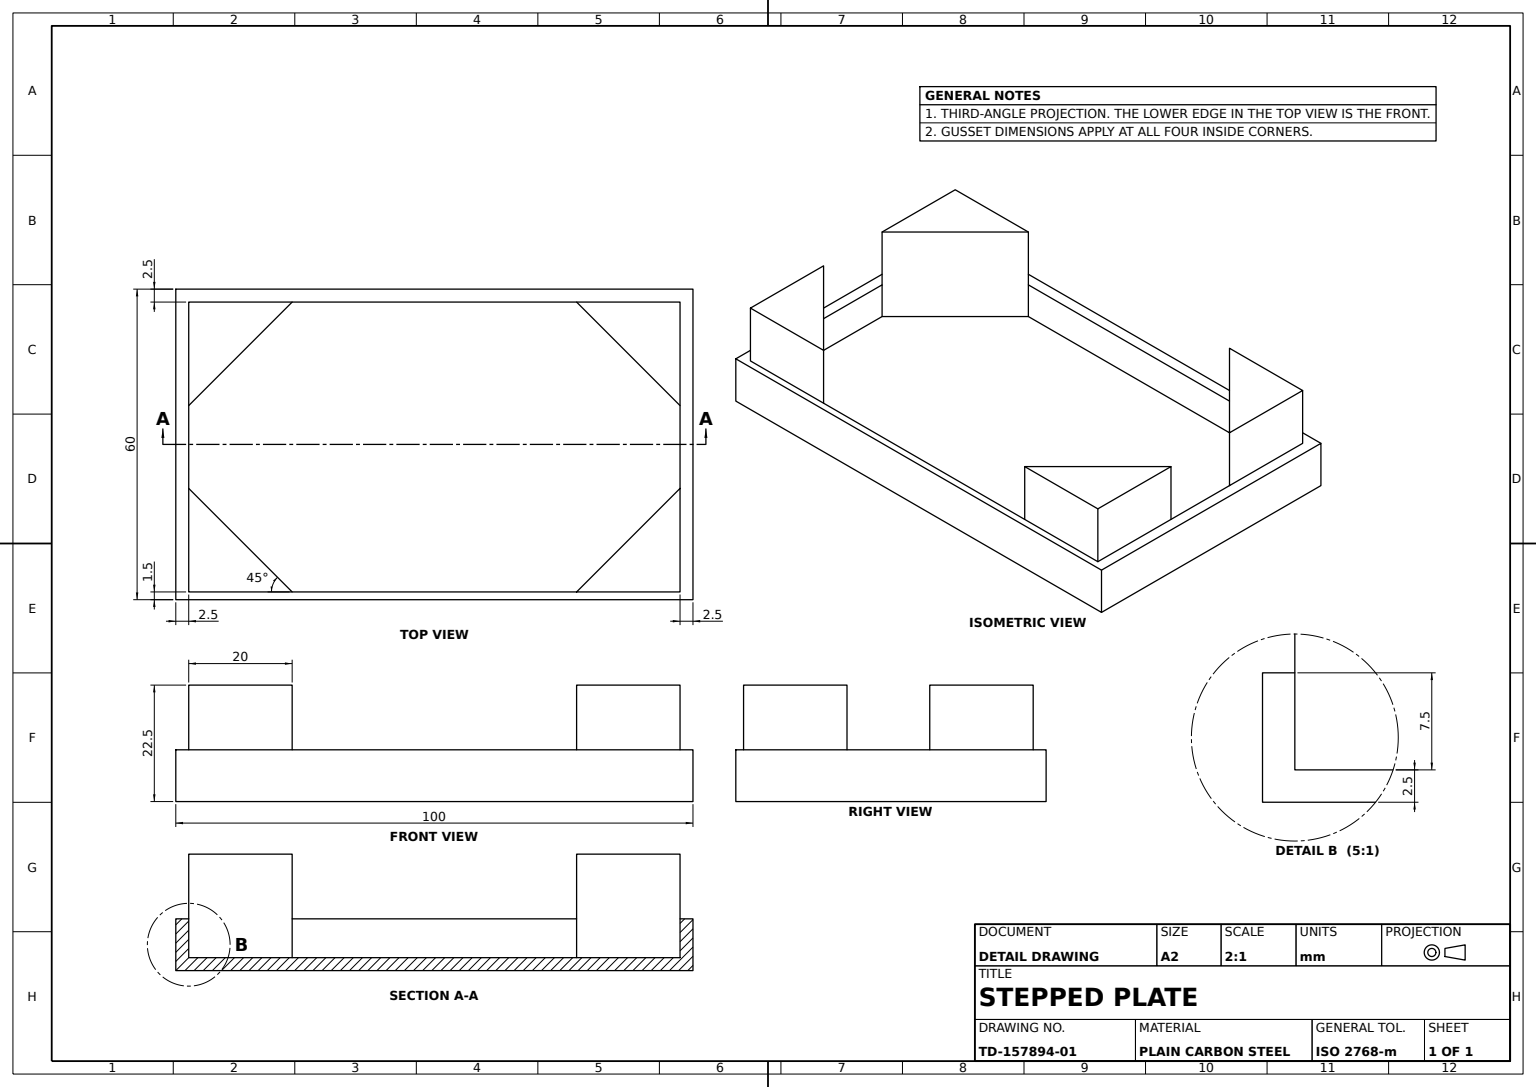
SolidWorks part; units mm, degrees
material "Plain Carbon Steel"
ref_plane "Front Plane" through (0, 0, 0) normal (0, 0, 1) x (1, 0, 0)
ref_plane "Top Plane" through (0, 0, 0) normal (0, 1, 0) x (1, 0, 0)
ref_plane "Right Plane" through (0, 0, 0) normal (1, 0, 0) x (0, 0, -1)
sketch "Base Plate Profile" plane through (0, 0, 0) normal (0, 0, 1) x (1, 0, 0)
  line L1 (0, 0) -> (100, 0)
  line L2 (0, 0) -> (0, 60)
  line L3 (0, 60) -> (100, 60)
  line L4 (100, 0) -> (100, 60)
  dimension "D1" = 100
  dimension "D2" = 60
extrude "Base Plate 2.5mm" add sketch "Base Plate Profile" along normal blind 2.5
sketch "Rim Wall Profile" plane through (0, 0, 2.5) normal (0, 0, 1) x (1, 0, 0)
  line L0 (100, 60) -> (0, 60) construction
  line L1 (0, 60) -> (100, 60)
  line L2 (0, 60) -> (0, 0)
  line L3 (0, 0) -> (100, 0)
  line L4 (100, 60) -> (100, 0)
  line L5 (0, 60) -> (100, 0) construction
  line L6 (0, 0) -> (100, 60) construction
  line L7 (0, 0) -> (100, 0) construction
  line L8 (0, 60) -> (0, 0) construction
  line L9 (100, 0) -> (100, 60) construction
  line L11 (2.5, 57.5) -> (97.5, 57.5)
  line L12 (2.5, 57.5) -> (2.5, 1.5)
  line L13 (2.5, 1.5) -> (97.5, 1.5)
  line L14 (97.5, 57.5) -> (97.5, 1.5)
  line L15 (2.5, 57.5) -> (97.5, 1.5) construction
  line L16 (2.5, 1.5) -> (97.5, 57.5) construction
  point P0 (50, 30)
  point P13 (50, 30)
  dimension "D1" = 2.5
  dimension "D2" = 2.5
  dimension "D3" = 2.5
extrude "Rim Wall 7.5mm" add sketch "Rim Wall Profile" along normal blind 7.5
sketch "Corner Gusset Profile" plane through (0, 0, 2.5) normal (0, 0, 1) x (1, 0, 0)
  line L0 (2.5, 57.5) -> (22.5, 57.5)
  line L1 (97.5, 57.5) -> (2.5, 57.5) construction
  line L2 (2.5, 57.5) -> (2.5, 37.5)
  line L3 (2.5, 57.5) -> (2.5, 1.5) construction
  line L4 (2.5, 37.5) -> (22.5, 57.5)
  line L5 (2.5, 1.5) -> (22.5, 1.5)
  line L6 (2.5, 1.5) -> (97.5, 1.5) construction
  line L7 (2.5, 1.5) -> (97.5, 1.5) construction
  line L8 (2.5, 1.5) -> (2.5, 21.5)
  line L9 (2.5, 21.5) -> (22.5, 1.5)
  line L10 (97.5, 57.5) -> (77.5, 57.5)
  line L11 (97.5, 57.5) -> (2.5, 57.5) construction
  line L12 (97.5, 57.5) -> (97.5, 37.5)
  line L13 (97.5, 1.5) -> (97.5, 57.5) construction
  line L14 (97.5, 37.5) -> (77.5, 57.5)
  line L15 (97.5, 1.5) -> (77.5, 1.5)
  line L16 (97.5, 1.5) -> (97.5, 21.5)
  line L17 (97.5, 21.5) -> (77.5, 1.5)
  dimension "D1" = 20
extrude "Corner Gussets 20mm" add sketch "Corner Gusset Profile" along normal blind 20
